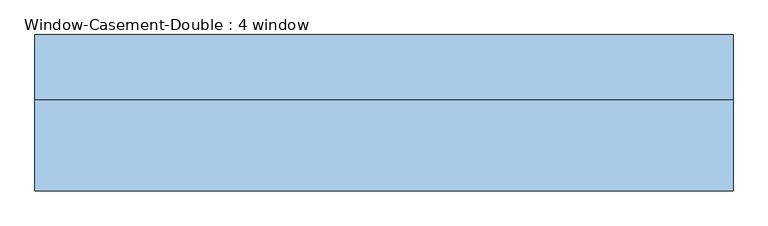
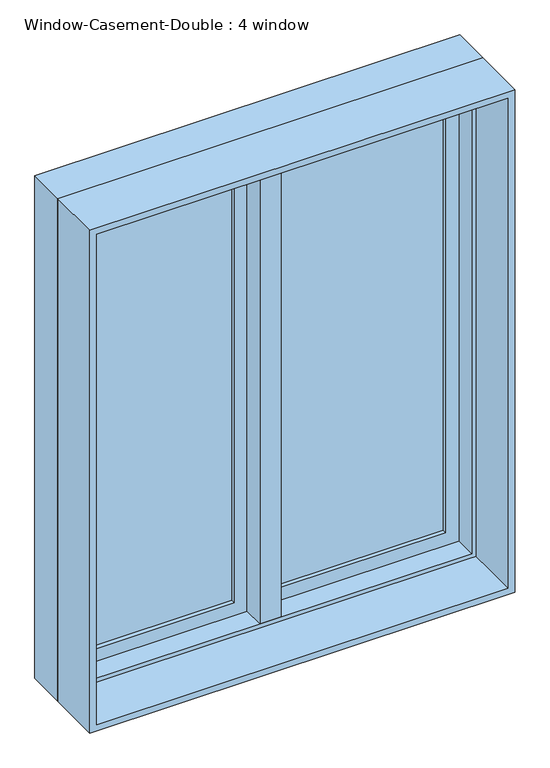
"""IFC4 building model written with IfcOpenShell, lengths in millimetres: window geometry, Window-Casement-Double : 4 window."""

from ifc_helpers import new_model, si_unit, frame, origin, place, context, project, spatial, polyline, outline, extrude, faceted_brep, source, transform, mapped, element, save


def window_casement_double_4_window_a93ed6b4(model_context):
    return source(origin(), model_context, "Body", "SolidModel", [
        faceted_brep([(9.525, 146.05, 2425.7), (-9.525, 146.05, 2425.7), (-9.525, 95.25, 2425.7), (9.525, 95.25, 2425.7), (9.525, 146.05, 927.1), (9.525, 95.25, 927.1), (-9.525, 95.25, 927.1), (-9.525, 146.05, 927.1), (-9.525, 95.25, 946.15), (-9.525, 95.25, 2406.65), (-30.1625, 95.25, 946.15), (-30.1625, 95.25, 2406.65), (-30.1625, 31.75, 946.15), (-30.1625, 31.75, 2406.65), (30.1625, 31.75, 946.15), (30.1625, 31.75, 2406.65), (30.1625, 95.25, 946.15), (30.1625, 95.25, 2406.65), (9.525, 95.25, 946.15), (9.525, 95.25, 2406.65)], [[[0, 1, 2, 3]], [[4, 5, 6, 7]], [[1, 0, 4, 7]], [[2, 1, 7, 6, 8, 9]], [[9, 8, 10, 11]], [[11, 10, 12, 13]], [[13, 12, 14, 15]], [[15, 14, 16, 17]], [[17, 16, 18, 19]], [[0, 3, 19, 18, 5, 4]], [[18, 8, 6, 5]], [[9, 19, 3, 2]], [[8, 18, 16, 14, 12, 10]], [[19, 9, 11, 13, 15, 17]]]),
        extrude(outline(polyline([(-66.675, 127.0), (-66.675, 120.65), (-539.75, 120.65), (-539.75, 127.0), (-66.675, 127.0)])), frame((0.0, 0.0, 984.25), z_axis=(0.0, 0.0, 1.0), x_axis=(1.0, 0.0, 0.0)), (0.0, 0.0, 1.0), 1384.3),
        extrude(outline(polyline([(-539.75, 107.95), (-539.75, 114.3), (-66.675, 114.3), (-66.675, 107.95), (-539.75, 107.95)])), frame((0.0, 0.0, 984.25), z_axis=(0.0, 0.0, 1.0), x_axis=(1.0, 0.0, 0.0)), (0.0, 0.0, 1.0), 1384.3),
        extrude(outline(polyline([(539.75, 127.0), (539.75, 120.65), (66.675, 120.65), (66.675, 127.0), (539.75, 127.0)])), frame((0.0, 0.0, 984.25), z_axis=(0.0, 0.0, 1.0), x_axis=(1.0, 0.0, 0.0)), (0.0, 0.0, 1.0), 1384.3),
        extrude(outline(polyline([(66.675, 107.95), (66.675, 114.3), (539.75, 114.3), (539.75, 107.95), (66.675, 107.95)])), frame((0.0, 0.0, 984.25), z_axis=(0.0, 0.0, 1.0), x_axis=(1.0, 0.0, 0.0)), (0.0, 0.0, 1.0), 1384.3),
        extrude(outline(polyline([(2425.7, -596.9), (927.1, -596.9), (927.1, -9.525), (2425.7, -9.525), (2425.7, -596.9)]), holes=[polyline([(2368.55, -66.675), (984.25, -66.675), (984.25, -539.75), (2368.55, -539.75), (2368.55, -66.675)])]), frame((0.0, 95.25, 0.0), z_axis=(0.0, 1.0, 0.0), x_axis=(0.0, 0.0, 1.0)), (0.0, 0.0, 1.0), 44.45),
        extrude(outline(polyline([(927.1, 596.9), (2425.7, 596.9), (2425.7, 9.525), (927.1, 9.525), (927.1, 596.9)]), holes=[polyline([(984.25, 66.675), (2368.55, 66.675), (2368.55, 539.75), (984.25, 539.75), (984.25, 66.675)])]), frame((0.0, 95.25, 0.0), z_axis=(0.0, 1.0, 0.0), x_axis=(0.0, 0.0, 1.0)), (0.0, 0.0, 1.0), 44.45),
        extrude(outline(polyline([(2438.4, -609.6), (914.4, -609.6), (914.4, 609.6), (2438.4, 609.6), (2438.4, -609.6)]), holes=[polyline([(2419.35, 590.55), (933.45, 590.55), (933.45, -590.55), (2419.35, -590.55), (2419.35, 590.55)])]), frame((0.0, -127.0, 0.0), z_axis=(0.0, 1.0, 0.0), x_axis=(0.0, 0.0, 1.0)), (0.0, 0.0, 1.0), 158.75),
        faceted_brep([(577.85, 95.25, 2406.65), (577.85, 31.75, 2406.65), (-577.85, 31.75, 2406.65), (-577.85, 95.25, 2406.65), (596.9, 146.05, 2425.7), (596.9, 95.25, 2425.7), (-596.9, 95.25, 2425.7), (-596.9, 146.05, 2425.7), (609.6, 31.75, 2438.4), (609.6, 146.05, 2438.4), (-609.6, 146.05, 2438.4), (-609.6, 31.75, 2438.4), (-577.85, 31.75, 946.15), (-577.85, 95.25, 946.15), (-596.9, 95.25, 927.1), (-596.9, 146.05, 927.1), (-609.6, 146.05, 914.4), (-609.6, 31.75, 914.4), (577.85, 31.75, 946.15), (577.85, 95.25, 946.15), (596.9, 95.25, 927.1), (596.9, 146.05, 927.1), (609.6, 146.05, 914.4), (609.6, 31.75, 914.4)], [[[0, 1, 2, 3]], [[4, 5, 6, 7]], [[8, 9, 10, 11]], [[3, 2, 12, 13]], [[7, 6, 14, 15]], [[11, 10, 16, 17]], [[13, 12, 18, 19]], [[15, 14, 20, 21]], [[17, 16, 22, 23]], [[11, 17, 23, 8], [1, 18, 12, 2]], [[19, 18, 1, 0]], [[5, 20, 14, 6], [3, 13, 19, 0]], [[21, 20, 5, 4]], [[23, 22, 9, 8]], [[9, 22, 16, 10], [7, 15, 21, 4]]]),
    ])


if __name__ == "__main__":
    model = new_model("IFC4")
    model_context = context("Model", 3, world=origin())
    ifc_project = project(units=[si_unit("LENGTHUNIT", "METRE", prefix="MILLI")], contexts=[model_context])
    site = spatial("IfcSite", under=ifc_project)
    building = spatial("IfcBuilding", under=site)
    placement = place(None, origin())
    window_casement_double_4_window_shape = window_casement_double_4_window_a93ed6b4(model_context)
    element("IfcWindow", 1, ObjectType="Window-Casement-Double : 4 window", at=placement, inside=building, context=model_context, shape_type="MappedRepresentation", body=[
        mapped(window_casement_double_4_window_shape, transform((0.0, 0.0, 0.0), x_axis=(1.0, 0.0, 0.0), y_axis=(0.0, 1.0, 0.0), z_axis=(0.0, 0.0, 1.0))),
    ])
    save(model, "model.ifc")

# Revit data of these elements
# Type "Window-Casement-Double : 4 window"
#   Type Mark = "21"
#   Fire Rating = "0.5h"
#   Assembly Code = "B2020100"
#   Analytic Construction = "Double glazing - domestic"
#   Frame Extension [instance default] = 0' - 0 1/4"
#   Window Inset [instance default] = 0' - 0"
#   Wall Thickness [instance default] = 0' - 6"
#   Interior Wall Closure [instance default] = 0' - 2 1/4"
#   Half Width = 2' - 0"
#   Visual Light Transmittance = 0.81
#   Thermal Resistance (R) = 1.8146 (h·ft²·°F)/BTU
#   Solar Heat Gain Coefficient = 0.76
#   Rough Width = 4' - 0 1/2"
#   Rough Height = 5' - 0 1/2"
#   Height = 5' - 0"
#   Heat Transfer Coefficient (U) = 0.5511 BTU/(h·ft²·°F)
#   Exterior Wall Closure [instance default] = 0' - 1 1/4"
#   Extension Jamb [instance default] = 0' - 2 1/4"
#   Default Sill Height = 3' - 0"
#   Width = 4' - 0"
#   Muntin Visibility = yes
#   Interior Trim Visibility [instance default] = yes
#   Exterior Trim Visibility [instance default] = yes
#   Extension Jamb Visibility [instance default] = yes
#   Interior Trim Material = Wood - Stained
#   Muntin Pattern = Muntin Pattern_2x2 : Muntin Pattern_2x2
#   Interior Trim = Trim-Window-Interior-Flat : Picture Frame
#   Interior Frame Material = Wood - Stained
#   Glass Panel Material = Glass
#   Exterior Trim Material = Clad - White
#   Exterior Trim = Trim-Window-Exterior-Flat : with Sill
#   Exterior Frame Material = Clad - White
#   Wall Closure = (empty or 0)
# Element 1 (IfcWindow, "Window-Casement-Double : 4 window")
#   Wall Thickness = 0' - 10"
#   Extension Jamb = 0' - 6 1/4"
#   Materials on its faces: "Wood - Stained", "Glass", "Clad - White"
# Materials
#   "Wood - Stained": class "Wood", colour RGB 224 178 126, transparency 0, Cost = 0
#   "Glass": class "Glass", colour RGB 0 128 192, transparency 0.75, Description = "Soda Lime Glass", Cost = 0
#   "Clad - White": class "Wood", colour RGB 242 242 238, transparency 0, Cost = 0
